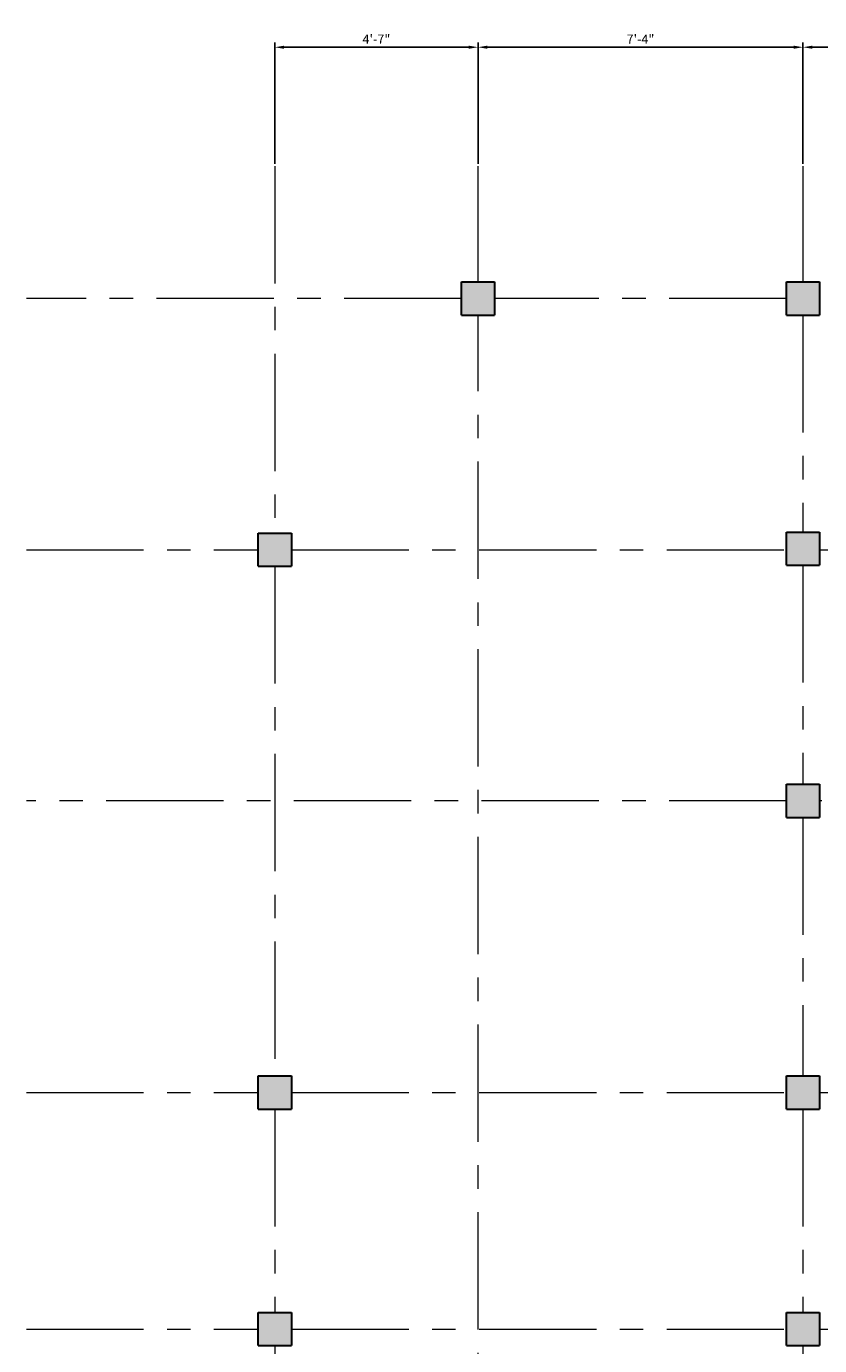
# Model space of a CAD drawing. Units: inches. Extents: x 4878 to 9282, y 5367 to 6617.
# Tile 8 of 14: x 5503 to 5718, y 6031 to 6388. Entities that reach past the tile are written whole.
import ezdxf

# ---------------------------------------------------------------- set-up
doc = ezdxf.new("R2010")
doc.units = ezdxf.units.IN
doc.linetypes.add('CENTER', pattern=[50.8, 31.75, -6.35, 6.35, -6.35])
for name, color, linetype, lineweight in [('A-ANNO-DIMS', 2, 'Continuous', 18), ('S-COLS', 1, 'Continuous', 30), ('S-COLS-PATT', 1, 'Continuous', 13), ('S-GRID', 4, 'CENTER', 13)]:
    doc.layers.add(name, color=color, linetype=linetype, lineweight=lineweight)
doc.styles.get("Standard").update_dxf_attribs({"font": 'arial.ttf'})
doc.dimstyles.new('ISO-25', dxfattribs={"dimtxt": 2.5, "dimasz": 2.5, "dimexe": 1.25, "dimexo": 0.625, "dimtad": 1, "dimdec": 0, "dimlunit": 3, "dimtxsty": 'Standard', "dimcen": 2.5, "dimadec": 0, "dimazin": 0, "dimtfac": 1, "dimtdec": 0, "dimtmove": 0, "dimatfit": 3, "dimfxl": 1, "dimarcsym": 0})

# ---------------------------------------------------------------- blocks, each defined once
blk = doc.blocks.new('COLUMN-9X9')
for p, q in [((0, 9), (9, 9)), ((0, 0), (0, 9)), ((9, 9), (9, 0)), ((0, 0), (9, 0))]:
    blk.add_line(p, q)
blk = doc.blocks.new('*D65')
at = {"layer": 'A-ANNO-DIMS', "color": 0, "lineweight": -2, "transparency": 16777216}
for p, q in [((5570.69, 6350.62), (5570.69, 6383.45)), ((5625.69, 6350.62), (5625.69, 6383.45)), ((5573.19, 6382.2), (5623.19, 6382.2))]:
    blk.add_line(p, q, dxfattribs=at)
at = {"layer": 'A-ANNO-DIMS', "color": 0, "transparency": 16777216}
for points in [[(5573.19, 6382.62), (5573.19, 6381.78), (5570.69, 6382.2)], [(5623.19, 6382.62), (5623.19, 6381.78), (5625.69, 6382.2)]]:
    blk.add_solid(points, dxfattribs=at)
at = {"layer": 'Defpoints', "color": 0, "transparency": 16777216}
for p in [(5625.69, 6382.2), (5570.69, 6350), (5625.69, 6350)]:
    blk.add_point(p, dxfattribs=at)
at = {"layer": 'A-ANNO-DIMS', "color": 0, "transparency": 16777216, "insert": (5598.19, 6384.07), "char_height": 2.5, "attachment_point": 5}
blk.add_mtext('4\'-7"', dxfattribs=at)
blk = doc.blocks.new('*D66')
at = {"layer": 'A-ANNO-DIMS', "color": 0, "lineweight": -2, "transparency": 16777216}
for p, q in [((5625.69, 6350.62), (5625.69, 6383.45)), ((5713.69, 6350.62), (5713.69, 6383.45)), ((5628.19, 6382.2), (5711.19, 6382.2))]:
    blk.add_line(p, q, dxfattribs=at)
at = {"layer": 'A-ANNO-DIMS', "color": 0, "transparency": 16777216}
for points in [[(5628.19, 6382.62), (5628.19, 6381.78), (5625.69, 6382.2)], [(5711.19, 6382.62), (5711.19, 6381.78), (5713.69, 6382.2)]]:
    blk.add_solid(points, dxfattribs=at)
at = {"layer": 'Defpoints', "color": 0, "transparency": 16777216}
for p in [(5713.69, 6382.2), (5625.69, 6350), (5713.69, 6350)]:
    blk.add_point(p, dxfattribs=at)
at = {"layer": 'A-ANNO-DIMS', "color": 0, "transparency": 16777216, "insert": (5669.69, 6384.07), "char_height": 2.5, "attachment_point": 5}
blk.add_mtext('7\'-4"', dxfattribs=at)
blk = doc.blocks.new('*D67')
at = {"layer": 'A-ANNO-DIMS', "color": 0, "lineweight": -2, "transparency": 16777216}
for p, q in [((5713.69, 6350.62), (5713.69, 6383.45)), ((5812.19, 6350.62), (5812.19, 6383.45)), ((5716.19, 6382.2), (5809.69, 6382.2))]:
    blk.add_line(p, q, dxfattribs=at)
at = {"layer": 'A-ANNO-DIMS', "color": 0, "transparency": 16777216}
for points in [[(5716.19, 6382.62), (5716.19, 6381.78), (5713.69, 6382.2)], [(5809.69, 6382.62), (5809.69, 6381.78), (5812.19, 6382.2)]]:
    blk.add_solid(points, dxfattribs=at)
at = {"layer": 'Defpoints', "color": 0, "transparency": 16777216}
for p in [(5812.19, 6382.2), (5713.69, 6350), (5812.19, 6350)]:
    blk.add_point(p, dxfattribs=at)
at = {"layer": 'A-ANNO-DIMS', "color": 0, "transparency": 16777216, "insert": (5762.94, 6384.12), "char_height": 2.5, "attachment_point": 5}
blk.add_mtext('8\'-2 1/2"', dxfattribs=at)

msp = doc.modelspace()

# ---------------------------------------------------------------- hatches: boundary and pattern name
at = {"layer": 'S-COLS-PATT'}
h = msp.add_hatch(color=256, dxfattribs=at)
h.dxf.hatch_style = 1
h.paths.add_polyline_path([(5621.19, 6309.64), (5630.19, 6309.64), (5630.19, 6318.64), (5621.19, 6318.64)])
h.paths.add_polyline_path([(5718.19, 6318.64), (5709.19, 6318.64), (5709.19, 6309.64), (5718.19, 6309.64)])
h.paths.add_polyline_path([(5575.19, 6241.64), (5575.19, 6250.64), (5566.19, 6250.64), (5566.19, 6241.64)])
h.paths.add_polyline_path([(5709.19, 6241.92), (5718.19, 6241.92), (5718.19, 6250.92), (5709.19, 6250.92)])
h.paths.add_polyline_path([(5816.69, 6250.64), (5807.69, 6250.64), (5807.69, 6241.64), (5816.69, 6241.64)])
h.paths.add_polyline_path([(5888.69, 6250.64), (5879.69, 6250.64), (5879.69, 6241.64), (5888.69, 6241.64)])
h.paths.add_polyline_path([(5964.69, 6250.64), (5955.69, 6250.64), (5955.69, 6241.64), (5964.69, 6241.64)])
h.paths.add_polyline_path([(5718.19, 6182.64), (5709.19, 6182.64), (5709.19, 6173.64), (5718.19, 6173.64)])
h.paths.add_polyline_path([(5816.69, 6182.64), (5807.69, 6182.64), (5807.69, 6173.64), (5816.69, 6173.64)])
h.paths.add_polyline_path([(5888.69, 6182.64), (5879.69, 6182.64), (5879.69, 6173.64), (5888.69, 6173.64)])
h.paths.add_polyline_path([(6013.69, 6173.64), (6022.69, 6173.64), (6022.69, 6182.64), (6013.69, 6182.64)])
h.paths.add_polyline_path([(6022.69, 6039.64), (6013.69, 6039.64), (6013.69, 6030.64), (6022.69, 6030.64)])
h.paths.add_polyline_path([(5879.69, 6030.64), (5888.69, 6030.64), (5888.69, 6039.64), (5879.69, 6039.64)])
h.paths.add_polyline_path([(5718.19, 6103.64), (5709.19, 6103.64), (5709.19, 6094.64), (5718.19, 6094.64)])
h.paths.add_polyline_path([(5718.19, 6039.64), (5709.19, 6039.64), (5709.19, 6030.64), (5718.19, 6030.64)])
h.paths.add_polyline_path([(5575.19, 6039.64), (5566.19, 6039.64), (5566.19, 6030.64), (5575.19, 6030.64)])
h.paths.add_polyline_path([(5566.19, 6094.64), (5575.19, 6094.64), (5575.19, 6103.64), (5566.19, 6103.64)])
h.paths.add_polyline_path([(5566.19, 5943.14), (5575.19, 5943.14), (5575.19, 5952.14), (5566.19, 5952.14)])
h.paths.add_polyline_path([(5575.19, 5864.64), (5566.19, 5864.64), (5566.19, 5855.64), (5575.19, 5855.64)])
h.paths.add_polyline_path([(5709.19, 5943.14), (5718.19, 5943.14), (5718.19, 5952.14), (5709.19, 5952.14)])
h.paths.add_polyline_path([(5718.19, 5855.64), (5718.19, 5864.64), (5709.19, 5864.64), (5709.19, 5855.64)])
h.paths.add_polyline_path([(5879.69, 5855.64), (5888.69, 5855.64), (5888.69, 5864.64), (5879.69, 5864.64)])
h.paths.add_polyline_path([(6013.69, 5855.64), (6022.69, 5855.64), (6022.69, 5864.64), (6013.69, 5864.64)])
h.paths.add_polyline_path([(5888.69, 5952.14), (5879.69, 5952.14), (5879.69, 5943.14), (5888.69, 5943.14)])

# ---------------------------------------------------------------- linework, layer by layer
at = {"layer": 'S-COLS'}
for p, q in [((5575.19, 6103.64), (5575.19, 6094.64)), ((5575.19, 6039.64), (5575.19, 6030.64))]:
    msp.add_line(p, q, dxfattribs=at)
at = {"layer": 'S-GRID'}
for p, q in [((5570.69, 6350), (5570.69, 6250.64)), ((5625.69, 6318.64), (5625.69, 6350)), ((5713.69, 6350), (5713.69, 6318.64)), ((5621.19, 6314.14), (5503.4, 6314.14)), ((5709.19, 6314.14), (5630.19, 6314.14)), ((5625.69, 5781.04), (5625.69, 6309.64)), ((5713.69, 6309.64), (5713.69, 6250.92)), ((5503.4, 6246.14), (5566.19, 6246.14)), ((5575.19, 6246.14), (5709.19, 6246.14)), ((5718.19, 6246.14), (5807.69, 6246.14)), ((5570.69, 6241.64), (5570.69, 6103.64)), ((5713.69, 6241.92), (5713.69, 6182.64)), ((5709.19, 6178.14), (5503.4, 6178.14)), ((5807.69, 6178.14), (5718.19, 6178.14)), ((5713.69, 6173.64), (5713.69, 6103.64)), ((5503.4, 6099.14), (5566.19, 6099.14)), ((5575.19, 6099.14), (5709.19, 6099.14)), ((5718.19, 6099.14), (6077.64, 6099.14)), ((5570.69, 6094.64), (5570.69, 6039.64)), ((5713.69, 6094.64), (5713.69, 6039.64)), ((5503.4, 6035.14), (5566.19, 6035.14)), ((5575.19, 6035.14), (5709.19, 6035.14)), ((5718.19, 6035.14), (5879.69, 6035.14)), ((5570.69, 6030.64), (5570.69, 5952.14)), ((5713.69, 6030.64), (5713.69, 5952.14))]:
    msp.add_line(p, q, dxfattribs=at)

# ---------------------------------------------------------------- block references
at = {"layer": 'S-COLS'}
for p in [(5621.19, 6309.65), (5709.19, 6309.65), (5566.19, 6241.65), (5709.19, 6241.92), (5709.19, 6173.65), (5566.19, 6094.65), (5709.19, 6094.65), (5566.19, 6030.65), (5709.19, 6030.65)]:
    msp.add_blockref('COLUMN-9X9', p, dxfattribs=at)

# ---------------------------------------------------------------- dimensions: what is measured, and where the dimension line sits
at = {"layer": 'A-ANNO-DIMS'}
for base, p1, p2, picture, middle in [((5812.19, 6382.2), (5713.69, 6350), (5812.19, 6350), '*D67', (5762.94, 6384.12)), ((5625.69, 6382.2), (5570.69, 6350), (5625.69, 6350), '*D65', (5598.19, 6384.07)), ((5713.69, 6382.2), (5625.69, 6350), (5713.69, 6350), '*D66', (5669.69, 6384.07))]:
    dim = msp.add_linear_dim(base=base, p1=p1, p2=p2, dimstyle='ISO-25', override={"dimdec": 1, "dimlfac": 1, "dimrnd": 0, "dimzin": 1, "dimdsep": 46, "dimlunit": 4, "dimfrac": 2}, dxfattribs=at)
    dim.commit()
    dim.dimension.update_dxf_attribs({"geometry": picture, "text_midpoint": middle})

doc.saveas('drawing.dxf')
